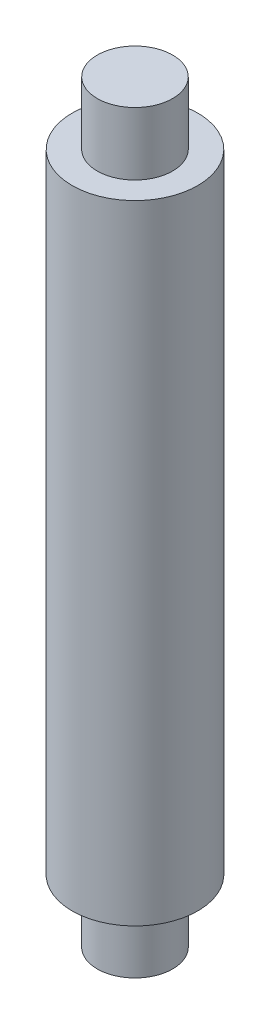
SolidWorks part; units mm, degrees
material "Plain Carbon Steel"
ref_plane "Front Plane" through (0, 0, 0) normal (0, 0, 1) x (1, 0, 0)
ref_plane "Top Plane" through (0, 0, 0) normal (0, 1, 0) x (1, 0, 0)
ref_plane "Right Plane" through (0, 0, 0) normal (1, 0, 0) x (0, 0, -1)
sketch "Shaft Profile Sketch" plane through (0, 0, 0) normal (0, 0, 1) x (1, 0, 0)
  line L0 (0, 0) -> (6, 0)
  line L1 (6, 0) -> (6, 10)
  line L2 (6, 10) -> (10, 10)
  line L3 (10, 10) -> (10, 110)
  line L4 (10, 110) -> (6, 110)
  line L5 (6, 110) -> (6, 120)
  line L6 (6, 120) -> (0, 120)
  line L7 (0, 120) -> (0, 0)
  dimension "D1" = 120
  dimension "D2" = 100
  dimension "D3" = 10
  dimension "D4" = 10
  dimension "D5" = 6
revolve "Stepped Shaft Ø20 Journals Ø12" add sketch "Shaft Profile Sketch" angle 360 about L7
